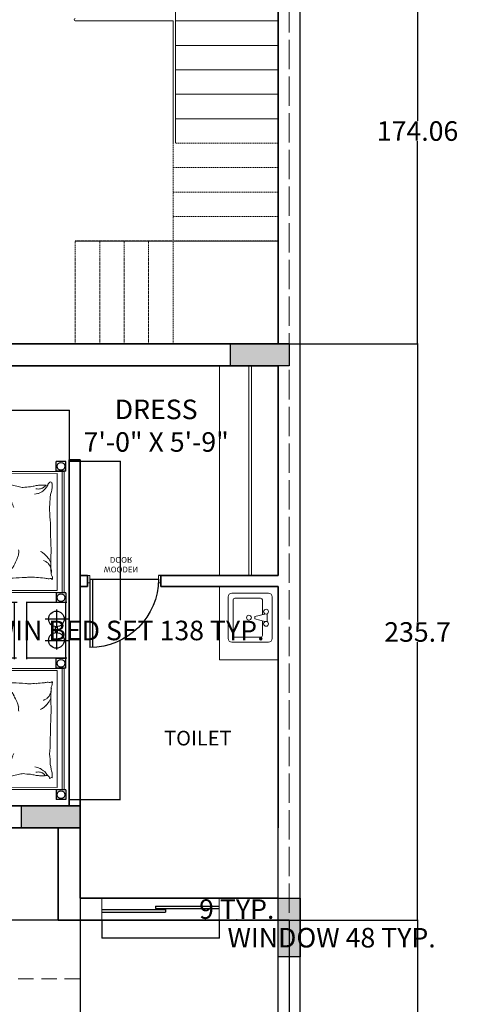
# Model space of a CAD drawing. Units: inches. Extents: x -48 to 50072, y 0 to 21068.
# Tile 53 of 75: x 439 to 618, y 417 to 819. Entities that reach past the tile are written whole.
import ezdxf

# ---------------------------------------------------------------- set-up
doc = ezdxf.new("R2010")
doc.units = ezdxf.units.IN
doc.header["$MEASUREMENT"] = 0
for name, pattern in [('ACAD_ISO02W100', [15, 12, -3]), ('DASHED', [0.75, 0.5, -0.25]), ('HIDDEN', [9.525, 6.35, -3.175])]:
    doc.linetypes.add(name, pattern=pattern)
for name, color, linetype, lineweight in [('A-ANNO-DIMS', 2, 'Continuous', 18), ('A-AREA-IDEN', 7, 'Continuous', 18), ('A-COLS', 1, 'Continuous', 35), ('A-DOOR', 4, 'Continuous', 18), ('A-FLOR-CASE', 9, 'Continuous', 18), ('A-FLOR-FIXT', 4, 'Continuous', 18), ('A-FLOR-OVHD', 8, 'HIDDEN', 13), ('A-FLOR-STRS', 7, 'Continuous', 18), ('A-FLOR-STRS-HIDN', 8, 'DASHED', 13), ('A-GLAZ', 4, 'Continuous', 18), ('A-WALL', 7, 'Continuous', 35), ('C-PROP', 7, 'Continuous', 25), ('C-PROP-REF', 32, 'ACAD_ISO02W100', 13), ('FURNITURE', 44, 'Continuous', 18)]:
    doc.layers.add(name, color=color, linetype=linetype, lineweight=lineweight)
for name, color, linetype in [('Layer3', 176, 'Continuous'), ('家具1', 1, 'Continuous'), ('家具１', 1, 'Continuous')]:
    doc.layers.add(name, color=color, linetype=linetype)
doc.styles.get("Standard").update_dxf_attribs({"font": 'arial.ttf'})
doc.dimstyles.get("Standard").update_dxf_attribs({"dimtxt": 8, "dimasz": 0.18, "dimexe": 0.18, "dimexo": 0.0625, "dimgap": 0.09, "dimtad": 0, "dimtih": 1, "dimtoh": 1, "dimdec": 1, "dimzin": 0, "dimdsep": 46, "dimlunit": 4, "dimtxsty": 'Standard', "dimblk": 'ARCHTICK', "dimcen": 0.09, "dimadec": 0, "dimazin": 0, "dimtfac": 1, "dimtdec": 1, "dimtofl": 0, "dimtmove": 0, "dimatfit": 3, "dimldrblk": 'ARCHTICK', "dimfxl": 1, "dimtolj": 1, "dimtzin": 0, "dimarcsym": 0})

# ---------------------------------------------------------------- blocks, each defined once
blk = doc.blocks.new('bnniku')
at = {"layer": 'Defpoints'}
h = blk.add_hatch(color=256, dxfattribs=at)
h.dxf.hatch_style = 1
h.paths.add_polyline_path([(767.55, 1114.04), (758.55, 1114.04), (758.55, 1090.04), (767.55, 1090.04)])
for p, q in [((758.55, 1114.04), (767.55, 1114.04)), ((758.55, 1090.04), (758.55, 1114.04)), ((767.55, 1114.04), (767.55, 1090.04)), ((767.55, 1090.04), (758.55, 1090.04))]:
    blk.add_line(p, q, dxfattribs=at)
blk = doc.blocks.new('gthyerhy')
at = {"layer": 'Defpoints'}
for p, q in [((665.59, 603.33), (665.59, 631.33)), ((666.59, 603.33), (666.59, 631.32)), ((665.59, 603.33), (693.59, 603.33))]:
    blk.add_line(p, q, dxfattribs=at)
blk.add_arc((665.59, 603.33), 28, 0, 90, dxfattribs=at)
at = {"insert": (674.82, 600.63), "char_height": 2.3647, "attachment_point": 1}
blk.add_mtext_dynamic_manual_height_columns('\\pxqc;WOODEN ^JDOOR', width=6.8949, gutter_width=11.82, heights=[0], dxfattribs=at)
blk = doc.blocks.new('gfhdr6777ju')
for p, q in [((466.52, 596.57), (467.52, 596.57)), ((467.52, 593.57), (467.52, 596.57)), ((495.52, 593.57), (495.52, 596.57)), ((466.52, 593.57), (467.52, 593.57)), ((495.52, 593.57), (496.52, 593.57))]:
    blk.add_line(p, q)
at = {"layer": 'Defpoints'}
blk.add_line((496.52, 596.57), (495.52, 596.57), dxfattribs=at)
at = {"layer": 'Defpoints', "xscale": -1, "rotation": 180}
blk.add_blockref('gthyerhy', (-198.07, 1198.41), dxfattribs=at)
blk = doc.blocks.new('windom')
for p, q in [((48.52, 1025.77), (48.52, 1034.77)), ((96.52, 1025.77), (96.52, 1034.77))]:
    blk.add_line(p, q)
at = {"layer": 'Defpoints'}
for p, q in [((70.52, 1031.47), (96.52, 1031.47)), ((70.52, 1031.47), (70.52, 1030.47)), ((48.52, 1030.07), (74.52, 1030.07)), ((48.52, 1029.07), (74.52, 1029.07)), ((70.52, 1030.47), (96.52, 1030.47)), ((74.52, 1030.07), (74.52, 1029.07))]:
    blk.add_line(p, q, dxfattribs=at)
at = {"layer": 'Layer3'}
for p, q in [((48.52, 1034.77), (96.52, 1034.77)), ((48.52, 1025.77), (96.52, 1025.77))]:
    blk.add_line(p, q, dxfattribs=at)
blk = doc.blocks.new('A$C7A8469D8')
for p, q in [((105, 2275), (1345, 2275)), ((105, 1661), (105, 2275)), ((1345, 2255), (105, 2255)), ((1345, 2275), (1345, 1540)), ((3364, 2275), (2124, 2275)), ((2124, 2275), (2124, 1540)), ((2124, 2255), (3364, 2255)), ((3364, 1661), (3364, 2275)), ((1325, 2205), (125, 2205)), ((129, 1663), (125, 2205)), ((1325, 1539), (1325, 2205)), ((2144, 2205), (3344, 2205)), ((2144, 1539), (2144, 2205)), ((3340, 1663), (3344, 2205)), ((941, 2062), (941, 2062)), ((964, 2087), (964, 2087)), ((964, 2087), (964, 2087)), ((997, 2116), (997, 2116)), ((2472, 2116), (2472, 2116)), ((2506, 2087), (2506, 2087)), ((2506, 2087), (2506, 2087)), ((2528, 2062), (2528, 2062)), ((284, 2013), (284, 2013)), ((284, 2013), (284, 2013)), ((3185, 2013), (3185, 2013)), ((3185, 2013), (3185, 2013)), ((240, 1733), (265, 1832)), ((3229, 1733), (3205, 1832)), ((231, 1697), (240, 1733)), ((1065, 1762), (1065, 1762)), ((1097, 1744), (1097, 1744)), ((1097, 1744), (1097, 1744)), ((1097, 1744), (1097, 1744)), ((2372, 1744), (2372, 1744)), ((2372, 1744), (2372, 1744)), ((2372, 1744), (2372, 1744)), ((2405, 1762), (2405, 1762)), ((3238, 1697), (3229, 1733)), ((1476, 1525), (6, 1701)), ((231, 1697), (230, 1695)), ((1993, 1525), (3463, 1701)), ((3238, 1697), (3239, 1695)), ((105, 212), (105, 1543)), ((125, 205), (125, 1562)), ((3344, 205), (3344, 1562)), ((3364, 212), (3364, 1543)), ((1325, 205), (1325, 1280)), ((1345, 1261), (1345, 212)), ((2124, 1261), (2124, 212)), ((2144, 205), (2144, 1280)), ((4, 94), (105, 212)), ((125, 205), (73, 144)), ((1325, 205), (1378, 144)), ((1345, 212), (1446, 92)), ((2124, 212), (2023, 92)), ((2144, 205), (2092, 144)), ((3344, 205), (3396, 144)), ((3465, 94), (3364, 212)), ((204, 30), (7, 169)), ((73, 144), (155, 88)), ((199, 135), (142, 0)), ((155, 88), (187, 155)), ((187, 155), (1264, 155)), ((1251, 135), (199, 135)), ((1453, 169), (1249, 34)), ((1324, 21), (1251, 135)), ((1296, 88), (1264, 155)), ((1378, 144), (1296, 88)), ((2017, 169), (2221, 34)), ((2092, 144), (2173, 88)), ((2145, 21), (2218, 135)), ((2173, 88), (2205, 155)), ((3282, 155), (2205, 155)), ((2218, 135), (3270, 135)), ((3265, 30), (3463, 169)), ((3270, 135), (3328, 0)), ((3315, 88), (3282, 155)), ((3396, 144), (3315, 88))]:
    blk.add_line(p, q)
for centre, radius, start, end in [((227, 2136), 15.7, 101.2724, 206.5805), ((250, 2148), 41, 206.5805, 265.5998), ((245, 2045), 108, 90, 101.2724), ((245, 1961), 193, 81.5628, 90), ((220, 1790), 366, 74.256, 81.5628), ((398, 2422), 291, 254.256, 262.4531), ((468, 2946), 819, 262.4531, 270), ((468, 3385), 1259, 270, 276.0867), ((201, 24611), 22481, 271.0184, 271.708), ((904, 1960), 183, 92.5386, 100.1899), ((911, 1796), 348, 85.1982, 92.5386), ((1028, 3186), 1048, 265.1982, 269.4243), ((1054, 2044), 92.1, 117.2396, 128.3886), ((1141, 1876), 281, 110.8603, 117.2396), ((1035, 3931), 1793, 269.4243, 271.9079), ((1130, 2026), 119, 126.0864, 143.8234), ((1130, 2026), 119, 105.9352, 126.0864), ((1062, 3124), 985, 271.9079, 275.2592), ((1130, 2026), 119, 85.7841, 105.9352), ((1147, 2207), 64.7, 275.2592, 300.6513), ((1197, 2122), 34.7, 85.6975, 120.6513), ((1198, 2126), 30.1, 68.2117, 85.6975), ((1220, 2138), 18.7, 158.0096, 201.421), ((1207, 2143), 5.13, 78.1069, 158.0096), ((1166, 2117), 39.3, 351.8665, 21.421), ((1209, 2151), 2.78, 258.1069, 19.564), ((1207, 2150), 4.1, 19.564, 68.2117), ((2257, 2156), 4.1, 291.7883, 340.436), ((2259, 2149), 2.78, 340.436, 101.8931), ((2258, 2184), 30.1, 274.3025, 291.7883), ((2266, 2150), 5.13, 201.9904, 281.8931), ((2228, 2126), 39.3, 338.579, 8.1335), ((2284, 2138), 18.7, 158.579, 201.9904), ((2287, 2186), 34.7, 239.3487, 274.3025), ((2284, 2087), 64.7, 59.3487, 84.7408), ((2284, 1158), 985, 84.7408, 88.0921), ((2363, 2260), 119, 254.0648, 274.2159), ((2442, 2237), 119, 233.9136, 254.0648), ((2392, 346), 1793, 88.0921, 90.5757), ((2505, 2193), 119, 216.1766, 233.9136), ((2557, 2388), 281, 242.7604, 249.1397), ((2540, 1094), 1048, 90.5757, 94.8018), ((2514, 2198), 92.1, 231.6114, 242.7604), ((2544, 2489), 348, 267.4614, 274.8018), ((2606, 2323), 183, 259.8101, 267.4614), ((2198, -20338), 22481, 88.292, 88.9816), ((2868, 875), 1259, 83.9133, 90), ((3109, 1314), 819, 90, 97.5469), ((3188, 1854), 291, 97.5469, 105.744), ((3096, 2504), 366, 278.4372, 285.744), ((3196, 2345), 193, 270, 278.4372), ((3259, 2088), 41, 94.4002, 153.4195), ((3245, 2260), 108, 258.7276, 270), ((3259, 2145), 15.7, 153.4195, 258.7276), ((833, 2043), 590, 173.7676, 180), ((488, 2043), 245, 180, 189.6844), ((181, 2001), 108, 41.4429, 53.7359), ((170, 1957), 168, 45.0976, 62.7964), ((214, 2030), 63.1, 25.3551, 41.4429), ((108, 1980), 181, 21.8149, 25.3551), ((47, 1955), 247, 18.7799, 21.8149), ((217, 2013), 67.4, 0, 18.7799), ((170, 1957), 168, 27.3988, 45.0976), ((170, 1957), 168, 16.515, 27.3988), ((1146, 1939), 240, 151.6832, 156.9972), ((987, 2024), 59.2, 140.9651, 151.6832), ((1151, 1892), 270, 133.8115, 140.9651), ((1151, 1892), 270, 133.8115, 140.9651), ((1151, 1892), 270, 133.8115, 140.9651), ((1289, 1747), 470, 128.3886, 133.8115), ((1289, 1747), 470, 128.3886, 133.8115), ((1289, 1747), 470, 128.3886, 133.8115), ((1130, 2026), 119, 143.8234, 161.5603), ((2284, 1927), 1096, 172.3191, 176.6313), ((1434, 2041), 238, 167.8905, 172.3191), ((912, 2153), 295, 347.8905, 351.8665), ((1976, 2049), 295, 8.1335, 12.1095), ((2504, 2123), 238, 187.6809, 192.1095), ((3365, 2137), 1096, 183.3687, 187.6809), ((2548, 2134), 119, 198.4397, 216.1766), ((2798, 2455), 470, 226.1885, 231.6114), ((2180, 1747), 470, 46.1885, 51.6114), ((2180, 1747), 470, 46.1885, 51.6114), ((2716, 2257), 270, 219.0349, 226.1885), ((2319, 1892), 270, 39.0349, 46.1885), ((2319, 1892), 270, 39.0349, 46.1885), ((2581, 2090), 59.2, 208.3168, 219.0349), ((2756, 2146), 240, 203.0028, 208.3168), ((2990, 2082), 168, 332.6012, 343.485), ((3032, 2154), 168, 314.9024, 332.6012), ((3104, 2226), 168, 297.2036, 314.9024), ((3121, 2035), 67.4, 341.2201, 360), ((2960, 2126), 247, 338.1851, 341.2201), ((3030, 2125), 181, 334.6449, 338.1851), ((3151, 2099), 63.1, 318.5571, 334.6449), ((3144, 2159), 108, 306.2641, 318.5571), ((3813, 2107), 590, 180, 186.2324), ((3468, 2002), 245, 170.3156, 180), ((1290, 2180), 1058, 189.6844, 192.1984), ((-117, 1876), 381, 8.0051, 12.1984), ((-523, 1819), 791, 2.6649, 8.0051), ((174, 2013), 110, 345.3149, 360), ((170, 1957), 168, 5.6311, 16.515), ((2003, 1943), 814, 176.6313, 181.6331), ((2826, 1967), 1638, 181.6331, 183.055), ((3094, 1968), 814, 178.3669, 183.3687), ((3917, 1833), 1638, 176.945, 178.3669), ((2972, 2022), 168, 343.485, 354.3689), ((3079, 1985), 110, 0, 14.6851), ((2419, 1966), 791, 351.9949, 357.3351), ((2837, 2009), 381, 347.8016, 351.9949), ((4257, 1778), 1058, 167.8016, 170.3156), ((186, 1852), 81.3, 345.9548, 2.6649), ((17530, 2751), 16363, 183.055, 183.5049), ((18611, 879), 16363, 176.4951, 176.945), ((3123, 1836), 81.3, 357.3351, 14.0452), ((-288, 1612), 350, 341.9888, 19.1136), ((93, 2561), 886, 287.1982, 289.428), ((93, 2561), 886, 289.4267, 291.8864), ((93, 2561), 886, 289.4283, 291.559), ((93, 2561), 886, 289.428, 291.6577), ((93, 2561), 886, 289.4267, 289.4283), ((93, 2561), 886, 291.443, 291.8345), ((93, 2561), 886, 291.43, 291.71), ((93, 2561), 886, 291.43, 291.7259), ((93, 2561), 886, 291.443, 291.484), ((93, 2561), 886, 291.484, 291.7259), ((93, 2561), 886, 291.559, 291.8345), ((93, 2561), 886, 291.6577, 293.4844), ((93, 2561), 886, 291.71, 291.8864), ((93, 2561), 886, 293.4844, 295.3111), ((1012, -5145), 6862, 89.7135, 90.9704), ((927, 1484), 326, 85.9172, 93.5552), ((946, 1740), 69.6, 69.3257, 85.9172), ((755, 1236), 608, 65.6735, 69.3257), ((298, 224), 1719, 63.5015, 65.6735), ((1040, 320), 1397, 86.426, 89.7135), ((897, 1427), 375, 57.865, 63.5015), ((897, 1427), 375, 57.865, 63.5015), ((897, 1427), 375, 57.865, 63.5015), ((632, 1004), 874, 54.1737, 57.865), ((1582, 1775), 385, 183.5049, 189.9984), ((2651, 1684), 385, 170.0016, 176.4951), ((1861, 2453), 874, 302.135, 305.8263), ((2335, 3111), 1397, 270.2865, 273.574), ((2205, 2080), 375, 296.4985, 302.135), ((2572, 1427), 375, 116.4985, 122.135), ((2572, 1427), 375, 116.4985, 122.135), ((1697, 3328), 1719, 294.3265, 296.4985), ((2539, 8578), 6862, 269.0296, 270.2865), ((2249, 2359), 608, 290.6743, 294.3265), ((2494, 1874), 69.6, 274.0828, 290.6743), ((2539, 2135), 326, 266.4448, 274.0828), ((2644, 947), 886, 64.6889, 66.5156), ((2696, 925), 886, 66.5156, 68.3423), ((3376, 2561), 886, 248.1136, 250.5733), ((3376, 2561), 886, 248.1136, 248.29), ((3376, 2561), 886, 248.1655, 248.557), ((3376, 2561), 886, 248.1655, 248.441), ((3376, 2561), 886, 248.29, 248.57), ((3376, 2561), 886, 248.2741, 248.57), ((3376, 2561), 886, 248.2741, 248.516), ((2754, 902), 886, 68.3423, 70.572), ((3376, 2561), 886, 248.441, 250.5717), ((3376, 2561), 886, 248.516, 248.557), ((3376, 2561), 886, 250.5717, 250.5733), ((2819, 879), 886, 70.572, 72.8018), ((3757, 1612), 350, 160.8864, 198.0112), ((209, 2020), 325, 273.8155, 274.0829), ((232, 1697), 1.1, 165.9546, 274.0829), ((232, 1697), 1.1, 165.9551, 274.0829), ((209, 2020), 325, 274.0829, 279.4841), ((217, 1971), 276, 279.4841, 287.3864), ((342, 1571), 144, 96.4341, 107.3864), ((346, 1540), 175, 78.4414, 96.4341), ((436, 1982), 276, 258.4414, 272.7491), ((369, 3390), 1686, 272.7491, 274.6176), ((622, 254), 1460, 92.6096, 94.6176), ((1098, -33471), 35188, 90.3285, 90.8836), ((1116, 1540), 175, 77.131, 86.426), ((1143, 1657), 54.3, 62.7159, 77.131), ((1210, 1788), 92.1, 242.7159, 253.7788), ((1214, 1800), 105, 253.7788, 262.8796), ((1201, 1697), 1.59, 262.8796, 343.3022), ((1180, 1704), 23.2, 343.3022, 9.9984), ((2244, 1701), 23.2, 350.0016, 16.6978), ((2267, 1695), 1.59, 16.6978, 97.1204), ((2298, 1595), 105, 97.1204, 106.2212), ((2327, 1617), 92.1, 106.2212, 117.2841), ((2289, 1759), 54.3, 282.869, 297.2841), ((2303, 1885), 175, 273.574, 282.869), ((3116, 36900), 35188, 269.1164, 269.6715), ((3031, 3168), 1460, 265.3824, 267.3904), ((2884, 26), 1686, 85.3824, 87.2509), ((3075, 1435), 276, 87.2509, 101.5586), ((3108, 1885), 175, 263.5659, 281.5586), ((3186, 1851), 144, 252.6136, 263.5659), ((3125, 1436), 276, 72.6136, 80.5159), ((3184, 1375), 325, 80.5159, 85.9171), ((3237, 1697), 1.1, 265.9171, 14.0454), ((3238, 1696), 1.1, 85.9171, 194.0449), ((3260, 2020), 325, 265.9171, 266.1845), ((192, -937), 2473, 57.4247, 94.4416), ((2297, 1493), 913, 173.1442, 204.7336), ((3278, -937), 2473, 85.5584, 122.5753), ((1172, 1493), 913, 335.2664, 6.8558)]:
    blk.add_arc(centre, radius, start, end)
at = {"layer": '家具1'}
for p, q in [((1614, 2082), (1614, 2330)), ((1836, 2082), (1836, 2330)), ((101, 2293), (1, 2293)), ((1, 2293), (1, 2193)), ((101, 2293), (101, 2193)), ((1348, 2293), (1448, 2293)), ((1348, 2293), (1348, 2193)), ((2032, 2293), (1441, 2293)), ((1448, 2303), (1448, 1885)), ((1448, 2293), (1448, 2193)), ((2018, 2303), (2018, 1885)), ((2121, 2293), (2021, 2293)), ((2021, 2293), (2021, 2193)), ((2121, 2293), (2121, 2193)), ((3369, 2293), (3469, 2293)), ((3369, 2293), (3369, 2193)), ((101, 2193), (1, 2193)), ((1348, 2193), (1448, 2193)), ((1518, 2197), (1709, 2197)), ((1757, 2206), (1696, 2206)), ((1757, 2186), (1696, 2186)), ((1741, 2197), (1931, 2197)), ((2121, 2193), (2021, 2193)), ((3369, 2193), (3469, 2193)), ((2029, 1893), (1441, 1893)), ((2029, 1768), (1441, 1768)), ((1448, 1793), (1448, 260)), ((2018, 1788), (2018, 260)), ((2029, 268), (1441, 268))]:
    blk.add_line(p, q, dxfattribs=at)
for centre, radius in [((51, 2243), 40), ((1398, 2243), 40), ((1616, 2196), 80), ((1836, 2196), 80), ((2071, 2243), 40), ((3419, 2243), 40)]:
    blk.add_circle(centre, radius, dxfattribs=at)
at = {"layer": '家具１'}
blk.add_line((3469, 2293), (3469, 2193), dxfattribs=at)
blk = doc.blocks.new('A$C329C6BD7')
at = {"linetype": 'ByBlock'}
for p, q in [((0, 0.419), (0, 0.038)), ((0.47, 0.457), (0.038, 0.457)), ((0.508, 0.038), (0.508, 0.419)), ((0.051, 0.07), (0.051, 0.337)), ((0.07, 0.356), (0.222, 0.356)), ((0.216, 0.406), (0.292, 0.406)), ((0.216, 0.381), (0.241, 0.279)), ((0.267, 0.279), (0.292, 0.381)), ((0.286, 0.356), (0.438, 0.356)), ((0.457, 0.337), (0.457, 0.07)), ((0.241, 0.279), (0.267, 0.279)), ((0.438, 0.051), (0.07, 0.051)), ((0.038, 0), (0.47, 0))]:
    blk.add_line(p, q, dxfattribs=at)
for centre in [(0.191, 0.394), (0.318, 0.394), (0.254, 0.216)]:
    blk.add_circle(centre, 0.0254, dxfattribs=at)
for centre, radius, start, end in [((0.038, 0.419), 0.0381, 90, 180), ((0.47, 0.419), 0.0381, 0, 90), ((0.07, 0.337), 0.0191, 90, 180), ((0.438, 0.337), 0.0191, 0, 90), ((0.038, 0.038), 0.0381, 180, 270), ((0.07, 0.07), 0.0191, 180, 270), ((0.438, 0.07), 0.0191, 270, 0), ((0.47, 0.038), 0.0381, 270, 0)]:
    blk.add_arc(centre, radius, start, end, dxfattribs=at)
blk = doc.blocks.new('_ArchTick')
at = {"color": 0, "linetype": 'ByBlock', "const_width": 0.15}
blk.add_lwpolyline([(-0.5, -0.5), (0.5, 0.5)], dxfattribs=at)
blk = doc.blocks.new('*D58')
at = {"layer": 'A-ANNO-DIMS', "color": 0, "lineweight": -2, "transparency": 16777216}
for p, q in [((472.35, 451.01), (472.35, 443.69)), ((520.35, 451.01), (520.35, 443.69)), ((472.35, 443.87), (520.35, 443.87)), ((520.35, 443.87), (520.53, 443.87))]:
    blk.add_line(p, q, dxfattribs=at)
at = {"layer": 'Defpoints', "color": 0, "transparency": 16777216}
for p in [(472.35, 451.07), (520.35, 451.07), (520.35, 443.87)]:
    blk.add_point(p, dxfattribs=at)
at = {"layer": 'A-ANNO-DIMS', "color": 0, "lineweight": -2, "transparency": 16777216, "xscale": 0.18, "yscale": 0.18, "zscale": 0.18, "rotation": 180}
blk.add_blockref('_ArchTick', (472.35, 443.87), dxfattribs=at)
at = {"layer": 'A-ANNO-DIMS', "color": 0, "lineweight": -2, "transparency": 16777216, "xscale": 0.18, "yscale": 0.18, "zscale": 0.18}
blk.add_blockref('_ArchTick', (520.35, 443.87), dxfattribs=at)
at = {"layer": 'A-ANNO-DIMS', "color": 0, "transparency": 16777216, "insert": (566.33, 443.87), "char_height": 8, "attachment_point": 5}
blk.add_mtext('\\A1;WINDOW 48 TYP.', dxfattribs=at)
blk = doc.blocks.new('*D59')
at = {"layer": 'A-ANNO-DIMS', "color": 0, "lineweight": -2, "transparency": 16777216}
for p, q in [((520.41, 460.07), (527.73, 460.07)), ((527.55, 460.07), (527.55, 459.75)), ((520.41, 451.07), (527.73, 451.07)), ((527.55, 451.07), (527.55, 451.4))]:
    blk.add_line(p, q, dxfattribs=at)
at = {"layer": 'Defpoints', "color": 0, "transparency": 16777216}
for p in [(520.35, 460.07), (527.55, 460.07), (520.35, 451.07)]:
    blk.add_point(p, dxfattribs=at)
at = {"layer": 'A-ANNO-DIMS', "color": 0, "lineweight": -2, "transparency": 16777216, "xscale": 0.18, "yscale": 0.18, "zscale": 0.18}
for p, rotation in [((527.55, 460.07), 90), ((527.55, 451.07), 270)]:
    blk.add_blockref('_ArchTick', p, dxfattribs=dict(at, rotation=rotation))
at = {"layer": 'A-ANNO-DIMS', "color": 0, "transparency": 16777216, "insert": (527.55, 455.57), "char_height": 8, "attachment_point": 5}
blk.add_mtext('\\A1;9 TYP.', dxfattribs=at)
blk = doc.blocks.new('*D74')
at = {"layer": 'A-ANNO-DIMS', "color": 0, "lineweight": -2, "transparency": 16777216}
for p, q in [((459.18, 638.72), (480.05, 638.72)), ((479.87, 638.72), (479.87, 573.76)), ((479.87, 500.35), (479.87, 565.3)), ((459.18, 500.35), (480.05, 500.35))]:
    blk.add_line(p, q, dxfattribs=at)
at = {"layer": 'Defpoints', "color": 0, "transparency": 16777216}
for p in [(459.12, 638.72), (459.12, 500.35), (479.87, 500.35)]:
    blk.add_point(p, dxfattribs=at)
at = {"layer": 'A-ANNO-DIMS', "color": 0, "lineweight": -2, "transparency": 16777216, "xscale": 0.18, "yscale": 0.18, "zscale": 0.18}
for p, rotation in [((479.87, 638.72), 90), ((479.87, 500.35), 270)]:
    blk.add_blockref('_ArchTick', p, dxfattribs=dict(at, rotation=rotation))
at = {"layer": 'A-ANNO-DIMS', "color": 0, "transparency": 16777216, "insert": (479.87, 569.53), "char_height": 8, "attachment_point": 5}
blk.add_mtext('\\A1;TWIN BED SET 138 TYP.', dxfattribs=at)
blk = doc.blocks.new('*D75')
at = {"layer": 'A-ANNO-DIMS', "color": 0, "lineweight": -2, "transparency": 16777216}
for p, q in [((366.2, 638.78), (366.2, 659.65)), ((366.2, 659.47), (393.1, 659.47)), ((459.12, 659.47), (432.22, 659.47)), ((459.12, 638.78), (459.12, 659.65))]:
    blk.add_line(p, q, dxfattribs=at)
at = {"layer": 'Defpoints', "color": 0, "transparency": 16777216}
for p in [(459.12, 659.47), (366.2, 638.72), (459.12, 638.72)]:
    blk.add_point(p, dxfattribs=at)
at = {"layer": 'A-ANNO-DIMS', "color": 0, "lineweight": -2, "transparency": 16777216, "xscale": 0.18, "yscale": 0.18, "zscale": 0.18, "rotation": 180}
blk.add_blockref('_ArchTick', (366.2, 659.47), dxfattribs=at)
at = {"layer": 'A-ANNO-DIMS', "color": 0, "lineweight": -2, "transparency": 16777216, "xscale": 0.18, "yscale": 0.18, "zscale": 0.18}
blk.add_blockref('_ArchTick', (459.12, 659.47), dxfattribs=at)
at = {"layer": 'A-ANNO-DIMS', "color": 0, "transparency": 16777216, "insert": (412.66, 659.47), "char_height": 8, "attachment_point": 5}
blk.add_mtext('\\A1;93 TYP.', dxfattribs=at)
blk = doc.blocks.new('*D115')
at = {"layer": 'A-ANNO-DIMS', "color": 0, "lineweight": -2, "transparency": 16777216}
for p, q in [((549.08, 451.07), (601.65, 451.07)), ((601.47, 451.07), (601.47, 336.75)), ((601.47, 214.07), (601.47, 328.4)), ((553.58, 214.07), (601.65, 214.07))]:
    blk.add_line(p, q, dxfattribs=at)
at = {"layer": 'Defpoints', "color": 0, "transparency": 16777216}
for p in [(549.02, 451.07), (601.47, 451.07), (553.52, 214.07)]:
    blk.add_point(p, dxfattribs=at)
at = {"layer": 'A-ANNO-DIMS', "color": 0, "lineweight": -2, "transparency": 16777216, "xscale": 0.18, "yscale": 0.18, "zscale": 0.18}
for p, rotation in [((601.47, 451.07), 90), ((601.47, 214.07), 270)]:
    blk.add_blockref('_ArchTick', p, dxfattribs=dict(at, rotation=rotation))
at = {"layer": 'A-ANNO-DIMS', "color": 0, "transparency": 16777216, "insert": (601.47, 332.57), "char_height": 8, "attachment_point": 5}
blk.add_mtext('\\A1;237', dxfattribs=at)
blk = doc.blocks.new('*D118')
at = {"layer": 'A-ANNO-DIMS', "color": 0, "lineweight": -2, "transparency": 16777216}
for p, q in [((297.02, 488.71), (297.02, 165.94)), ((463.52, 488.71), (463.52, 165.94)), ((297.02, 166.12), (367.03, 166.12)), ((463.52, 166.12), (393.51, 166.12))]:
    blk.add_line(p, q, dxfattribs=at)
at = {"layer": 'Defpoints', "color": 0, "transparency": 16777216}
for p in [(297.02, 488.77), (463.52, 488.77), (463.52, 166.12)]:
    blk.add_point(p, dxfattribs=at)
at = {"layer": 'A-ANNO-DIMS', "color": 0, "lineweight": -2, "transparency": 16777216, "xscale": 0.18, "yscale": 0.18, "zscale": 0.18, "rotation": 180}
blk.add_blockref('_ArchTick', (297.02, 166.12), dxfattribs=at)
at = {"layer": 'A-ANNO-DIMS', "color": 0, "lineweight": -2, "transparency": 16777216, "xscale": 0.18, "yscale": 0.18, "zscale": 0.18}
blk.add_blockref('_ArchTick', (463.52, 166.12), dxfattribs=at)
at = {"layer": 'A-ANNO-DIMS', "color": 0, "transparency": 16777216, "insert": (380.27, 166.12), "char_height": 8, "attachment_point": 5}
blk.add_mtext('\\A1;166.5', dxfattribs=at)
blk = doc.blocks.new('*D119')
at = {"layer": 'A-ANNO-DIMS', "color": 0, "lineweight": -2, "transparency": 16777216}
for p, q in [((463.52, 451.01), (463.52, 165.94)), ((549.02, 451.01), (549.02, 165.94)), ((463.52, 166.12), (495.75, 166.12)), ((549.02, 166.12), (516.78, 166.12))]:
    blk.add_line(p, q, dxfattribs=at)
at = {"layer": 'Defpoints', "color": 0, "transparency": 16777216}
for p in [(463.52, 451.07), (549.02, 451.07), (549.02, 166.12)]:
    blk.add_point(p, dxfattribs=at)
at = {"layer": 'A-ANNO-DIMS', "color": 0, "lineweight": -2, "transparency": 16777216, "xscale": 0.18, "yscale": 0.18, "zscale": 0.18, "rotation": 180}
blk.add_blockref('_ArchTick', (463.52, 166.12), dxfattribs=at)
at = {"layer": 'A-ANNO-DIMS', "color": 0, "lineweight": -2, "transparency": 16777216, "xscale": 0.18, "yscale": 0.18, "zscale": 0.18}
blk.add_blockref('_ArchTick', (549.02, 166.12), dxfattribs=at)
at = {"layer": 'A-ANNO-DIMS', "color": 0, "transparency": 16777216, "insert": (506.27, 166.12), "char_height": 8, "attachment_point": 5}
blk.add_mtext('\\A1;85.5', dxfattribs=at)
blk = doc.blocks.new('*D121')
at = {"layer": 'A-ANNO-DIMS', "color": 0, "lineweight": -2, "transparency": 16777216}
for p, q in [((549.08, 860.84), (601.65, 860.84)), ((601.47, 860.84), (601.47, 777.98)), ((601.47, 686.77), (601.47, 769.63)), ((549.08, 686.77), (601.65, 686.77))]:
    blk.add_line(p, q, dxfattribs=at)
at = {"layer": 'Defpoints', "color": 0, "transparency": 16777216}
for p in [(549.02, 860.84), (549.02, 686.77), (601.47, 686.77)]:
    blk.add_point(p, dxfattribs=at)
at = {"layer": 'A-ANNO-DIMS', "color": 0, "lineweight": -2, "transparency": 16777216, "xscale": 0.18, "yscale": 0.18, "zscale": 0.18}
for p, rotation in [((601.47, 860.84), 90), ((601.47, 686.77), 270)]:
    blk.add_blockref('_ArchTick', p, dxfattribs=dict(at, rotation=rotation))
at = {"layer": 'A-ANNO-DIMS', "color": 0, "transparency": 16777216, "insert": (601.47, 773.81), "char_height": 8, "attachment_point": 5}
blk.add_mtext('\\A1;174.06', dxfattribs=at)
blk = doc.blocks.new('*D122')
at = {"layer": 'A-ANNO-DIMS', "color": 0, "lineweight": -2, "transparency": 16777216}
for p, q in [((549.08, 686.77), (601.65, 686.77)), ((601.47, 686.77), (601.47, 573.1)), ((601.47, 451.07), (601.47, 564.75)), ((549.08, 451.07), (601.65, 451.07))]:
    blk.add_line(p, q, dxfattribs=at)
at = {"layer": 'Defpoints', "color": 0, "transparency": 16777216}
for p in [(549.02, 686.77), (549.02, 451.07), (601.47, 451.07)]:
    blk.add_point(p, dxfattribs=at)
at = {"layer": 'A-ANNO-DIMS', "color": 0, "lineweight": -2, "transparency": 16777216, "xscale": 0.18, "yscale": 0.18, "zscale": 0.18}
for p, rotation in [((601.47, 686.77), 90), ((601.47, 451.07), 270)]:
    blk.add_blockref('_ArchTick', p, dxfattribs=dict(at, rotation=rotation))
at = {"layer": 'A-ANNO-DIMS', "color": 0, "transparency": 16777216, "insert": (601.47, 568.92), "char_height": 8, "attachment_point": 5}
blk.add_mtext('\\A1;235.7', dxfattribs=at)
blk = doc.blocks.new('*D128')
at = {"layer": 'A-ANNO-DIMS', "color": 0, "lineweight": -2, "transparency": 16777216}
for p, q in [((463.45, 488.77), (-34.61, 488.77)), ((-34.43, 488.77), (-34.43, 474.1)), ((-34.43, 451.07), (-34.43, 465.75)), ((463.45, 451.07), (-34.61, 451.07))]:
    blk.add_line(p, q, dxfattribs=at)
at = {"layer": 'Defpoints', "color": 0, "transparency": 16777216}
for p in [(-34.43, 488.77), (463.52, 488.77), (463.52, 451.07)]:
    blk.add_point(p, dxfattribs=at)
at = {"layer": 'A-ANNO-DIMS', "color": 0, "lineweight": -2, "transparency": 16777216, "xscale": 0.18, "yscale": 0.18, "zscale": 0.18}
for p, rotation in [((-34.43, 488.77), 90), ((-34.43, 451.07), 270)]:
    blk.add_blockref('_ArchTick', p, dxfattribs=dict(at, rotation=rotation))
at = {"layer": 'A-ANNO-DIMS', "color": 0, "transparency": 16777216, "insert": (-34.43, 469.92), "char_height": 8, "attachment_point": 5}
blk.add_mtext('\\A1;37.7', dxfattribs=at)

msp = doc.modelspace()

# ---------------------------------------------------------------- linework, layer by layer
at = {"layer": 'A-FLOR-CASE'}
for p, q in [((520.517, 592.075), (520.517, 677.775)), ((532.517, 592.075), (532.517, 677.775)), ((533.517, 592.075), (533.517, 677.775)), ((520.517, 557.575), (520.517, 587.575)), ((520.517, 557.575), (544.517, 557.575))]:
    msp.add_line(p, q, dxfattribs=at)
at = {"layer": 'A-FLOR-OVHD'}
for p, q in [((463.517, 451.075), (463.517, 427.075)), ((463.517, 427.075), (296.953, 427.075))]:
    msp.add_line(p, q, dxfattribs=at)
at = {"layer": 'A-FLOR-STRS'}
for p, q in [((502.517, 768.838), (502.517, 860.838)), ((501.517, 818.838), (461.517, 818.838)), ((501.517, 768.838), (501.517, 818.838)), ((544.517, 818.838), (502.517, 818.838)), ((544.517, 808.838), (502.517, 808.838)), ((544.517, 798.838), (502.517, 798.838)), ((544.517, 788.838), (502.517, 788.838)), ((544.517, 778.838), (502.517, 778.838)), ((544.517, 728.775), (461.517, 728.775))]:
    msp.add_line(p, q, dxfattribs=at)
msp.add_arc((461.517, 819.338), 0.5, 90, 270, dxfattribs=at)
at = {"layer": 'A-FLOR-STRS-HIDN'}
for p, q in [((501.517, 768.838), (501.517, 686.838)), ((544.517, 768.838), (502.517, 768.838)), ((544.517, 758.838), (501.517, 758.838)), ((544.517, 748.838), (501.517, 748.838)), ((544.517, 738.838), (501.517, 738.838)), ((461.517, 686.838), (461.517, 728.838)), ((544.517, 728.838), (461.517, 728.838)), ((471.517, 686.838), (471.517, 728.838)), ((481.517, 686.838), (481.517, 728.838)), ((491.517, 686.838), (491.517, 728.838))]:
    msp.add_line(p, q, dxfattribs=at)
at = {"layer": 'A-WALL'}
for p, q in [((544.517, 686.775), (544.517, 860.838)), ((549.017, 686.775), (297.017, 686.775)), ((544.517, 677.775), (297.017, 677.775)), ((544.517, 592.075), (544.517, 677.775)), ((459.017, 497.775), (459.017, 639.367)), ((459.017, 639.367), (463.517, 639.367)), ((463.517, 592.075), (463.517, 639.367)), ((463.517, 460.075), (463.517, 592.075)), ((463.517, 592.075), (466.517, 592.075)), ((466.517, 587.575), (466.517, 592.075)), ((496.517, 587.575), (496.517, 592.075)), ((496.517, 592.075), (544.517, 592.075)), ((463.517, 587.575), (466.517, 587.575)), ((496.517, 587.575), (544.517, 587.575)), ((544.517, 488.775), (544.517, 587.575)), ((463.517, 497.775), (216.017, 497.775)), ((463.517, 488.775), (216.017, 488.775)), ((454.517, 451.075), (454.517, 488.775)), ((463.517, 460.075), (463.517, 488.775)), ((463.517, 460.075), (544.517, 460.075)), ((454.517, 451.075), (549.017, 451.075))]:
    msp.add_line(p, q, dxfattribs=at)
at = {"layer": 'C-PROP'}
for p, q in [((553.517, 214.075), (553.517, 1170.775)), ((544.517, 223.075), (544.517, 488.775))]:
    msp.add_line(p, q, dxfattribs=at)
at = {"layer": 'C-PROP-REF'}
msp.add_line((549.017, 214.075), (549.017, 1166.275), dxfattribs=at)

# ---------------------------------------------------------------- block references
at = {"layer": 'A-COLS'}
for p, rotation in [((1639.054, -80.777), 90), ((-650.52, 1256.326), 270)]:
    msp.add_blockref('bnniku', p, dxfattribs=dict(at, rotation=rotation))
msp.add_blockref('bnniku', (-214.034, -653.962), dxfattribs=at)
at = {"layer": 'A-DOOR'}
msp.add_blockref('gfhdr6777ju', (0, -4.5), dxfattribs=at)
at = {"layer": 'A-FLOR-FIXT', "xscale": 39.38263526611686, "yscale": 39.38263526611686, "zscale": 39.38263526611686, "rotation": 270}
msp.add_blockref('A$C329C6BD7', (524.01, 584.763), dxfattribs=at)
at = {"layer": 'A-GLAZ'}
msp.add_blockref('windom', (423.834, -574.7), dxfattribs=at)
at = {"layer": 'FURNITURE', "xscale": 0.0398840429945948, "yscale": 0.0398840429945948, "zscale": 0.0398840429945948, "rotation": 270}
msp.add_blockref('A$C7A8469D8', (366.197, 638.717), dxfattribs=at)

# ---------------------------------------------------------------- texts
at = {"layer": 'A-AREA-IDEN', "attachment_point": 1}
for s, width, gutter_width, insert, char_height in [('\\pxqc;DRESS^J7\'-0" X 5\'-9"', 128.05681, 40, (430.568, 663.964), 8), ('TOILET ', 46.2236, 30, (497.849, 528.508), 6)]:
    msp.add_mtext_dynamic_manual_height_columns(s, width=width, gutter_width=gutter_width, heights=[0], dxfattribs=dict(at, insert=insert, char_height=char_height))

# ---------------------------------------------------------------- dimensions: what is measured, and where the dimension line sits
at = {"layer": 'A-ANNO-DIMS'}
for base, p1, p2, override, picture, middle in [((601.467, 686.775), (549.017, 860.838), (549.017, 686.775), {"dimdec": 2, "dimlfac": 1, "dimrnd": 0, "dimzin": 0, "dimdsep": 46, "dimlunit": 2}, '*D121', (601.467, 773.806)), ((601.467, 451.075), (549.017, 686.775), (549.017, 451.075), {"dimdec": 1, "dimlfac": 1, "dimrnd": 0, "dimzin": 0, "dimdsep": 46, "dimlunit": 2}, '*D122', (601.467, 568.925)), ((-34.433, 488.775), (463.517, 451.075), (463.517, 488.775), {"dimdec": 1, "dimlfac": 1, "dimrnd": 0, "dimzin": 0, "dimdsep": 46, "dimlunit": 2}, '*D128', (-34.433, 469.925)), ((601.467, 451.075), (553.517, 214.075), (549.017, 451.075), {"dimdec": 0, "dimlfac": 1, "dimrnd": 0, "dimzin": 0, "dimdsep": 46, "dimlunit": 2}, '*D115', (601.467, 332.575))]:
    dim = msp.add_linear_dim(base=base, p1=p1, p2=p2, angle=90, dimstyle='Standard', override=override, dxfattribs=at)
    dim.commit()
    dim.dimension.update_dxf_attribs({"geometry": picture, "text_midpoint": middle})
for base, p1, p2, text, picture, middle in [((459.119, 659.472), (366.197, 638.717), (459.119, 638.717), '<> TYP.', '*D75', (412.658, 659.472)), ((520.351, 443.875), (472.351, 451.075), (520.351, 451.075), 'WINDOW <> TYP.', '*D58', (566.326, 443.875))]:
    dim = msp.add_linear_dim(base=base, p1=p1, p2=p2, text=text, dimstyle='Standard', override={"dimdec": 0, "dimlfac": 1, "dimrnd": 0, "dimzin": 0, "dimdsep": 46, "dimlunit": 2}, dxfattribs=at)
    dim.commit()
    dim.dimension.update_dxf_attribs({"geometry": picture, "text_midpoint": middle})
for base, p1, p2, angle, text, picture, middle in [((479.874, 500.347), (459.119, 638.717), (459.119, 500.347), 270, 'TWIN BED SET <> TYP.', '*D74', (479.874, 569.532)), ((527.551, 460.075), (520.351, 451.075), (520.351, 460.075), 90, '<> TYP.', '*D59', (527.551, 455.575))]:
    dim = msp.add_linear_dim(base=base, p1=p1, p2=p2, angle=angle, text=text, dimstyle='Standard', override={"dimdec": 0, "dimlfac": 1, "dimrnd": 0, "dimzin": 0, "dimdsep": 46, "dimlunit": 2}, dxfattribs=at)
    dim.commit()
    dim.dimension.update_dxf_attribs({"geometry": picture, "text_midpoint": middle})
for base, p1, p2, picture, middle in [((463.517, 166.125), (297.017, 488.775), (463.517, 488.775), '*D118', (380.267, 166.125)), ((549.017, 166.125), (463.517, 451.075), (549.017, 451.075), '*D119', (506.267, 166.125))]:
    dim = msp.add_linear_dim(base=base, p1=p1, p2=p2, dimstyle='Standard', override={"dimdec": 1, "dimlfac": 1, "dimrnd": 0, "dimzin": 0, "dimdsep": 46, "dimlunit": 2}, dxfattribs=at)
    dim.commit()
    dim.dimension.update_dxf_attribs({"geometry": picture, "text_midpoint": middle})

doc.saveas('drawing.dxf')
